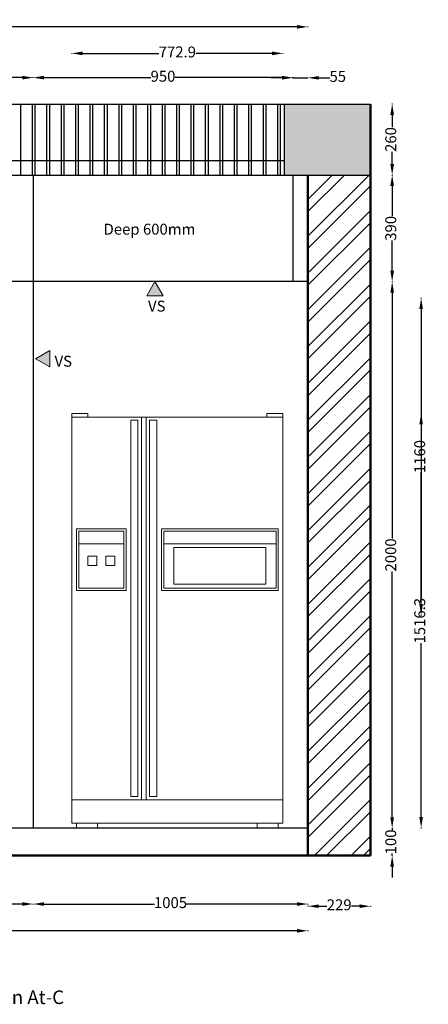
# Model space of a CAD drawing. Units: millimetres. Extents: x 2054 to 5837, y -782 to 2821.
# Tile 2 of 2: x 4342 to 5837, y -782 to 2821. Entities that reach past the tile are written whole.
import ezdxf

# ---------------------------------------------------------------- set-up
doc = ezdxf.new("R2010")
doc.units = ezdxf.units.MM
for name, color, linetype, lineweight in [('A-ANNO-DIMS', 2, 'Continuous', 18), ('A-ANNO-SYMB', 1, 'Continuous', 18), ('A-ANNO-TEXT', 7, 'Continuous', 18), ('A-EQPM', 8, 'Continuous', 18), ('A-FURN', 42, 'Continuous', 25), ('A-FURN-PATT', 8, 'Continuous', 13), ('A-WALL', 7, 'Continuous', 50), ('A-WALL-PATT', 8, 'Continuous', 13)]:
    doc.layers.add(name, color=color, linetype=linetype, lineweight=lineweight)
doc.styles.get("Standard").update_dxf_attribs({"font": 'arial.ttf'})
doc.dimstyles.new('ISO-25', dxfattribs={"dimtxt": 40, "dimasz": 40, "dimexe": 1.25, "dimexo": 0.625, "dimtad": 0, "dimtxsty": 'Standard', "dimcen": 2.5, "dimclrt": 1, "dimadec": 0, "dimazin": 0, "dimtfac": 1, "dimtmove": 0, "dimatfit": 3, "dimfxl": 1, "dimfxlon": 1, "dimarcsym": 0})

# ---------------------------------------------------------------- blocks, each defined once
blk = doc.blocks.new('*D1')
at = {"layer": 'A-ANNO-DIMS', "color": 0, "lineweight": -2, "transparency": 16777216}
for p, q in [((4391.1, -414.1), (4391.1, -416.4)), ((4431.1, -415.1), (4835, -415.1)), ((5356.1, -415.1), (4952.2, -415.1)), ((5396.1, -414.1), (5396.1, -416.4))]:
    blk.add_line(p, q, dxfattribs=at)
at = {"layer": 'A-ANNO-DIMS', "color": 0, "transparency": 16777216}
for points in [[(4431.1, -408.4), (4431.1, -421.8), (4391.1, -415.1)], [(5356.1, -408.4), (5356.1, -421.8), (5396.1, -415.1)]]:
    blk.add_solid(points, dxfattribs=at)
at = {"layer": 'Defpoints', "color": 0, "transparency": 16777216}
for p in [(4391.1, -137.8), (5396.1, -137.8), (4391.1, -415.1)]:
    blk.add_point(p, dxfattribs=at)
at = {"layer": 'A-ANNO-DIMS', "color": 0, "transparency": 16777216, "insert": (4893.6, -415.1), "char_height": 40, "attachment_point": 5}
blk.add_mtext('1005', dxfattribs=at)
blk = doc.blocks.new('*D2')
at = {"layer": 'A-ANNO-DIMS', "color": 0, "lineweight": -2, "transparency": 16777216}
for p, q in [((3941.1, -414.1), (3941.1, -416.4)), ((3981.1, -415.1), (4120.6, -415.1)), ((4351.1, -415.1), (4211.7, -415.1)), ((4391.1, -414.1), (4391.1, -416.4))]:
    blk.add_line(p, q, dxfattribs=at)
at = {"layer": 'A-ANNO-DIMS', "color": 0, "transparency": 16777216}
for points in [[(3981.1, -408.4), (3981.1, -421.8), (3941.1, -415.1)], [(4351.1, -408.4), (4351.1, -421.8), (4391.1, -415.1)]]:
    blk.add_solid(points, dxfattribs=at)
at = {"layer": 'Defpoints', "color": 0, "transparency": 16777216}
for p in [(3941.1, -137.8), (4391.1, -137.8), (3941.1, -415.1)]:
    blk.add_point(p, dxfattribs=at)
at = {"layer": 'A-ANNO-DIMS', "color": 0, "transparency": 16777216, "insert": (4166.1, -415.1), "char_height": 40, "attachment_point": 5}
blk.add_mtext('450', dxfattribs=at)
blk = doc.blocks.new('*D6')
at = {"layer": 'A-ANNO-DIMS', "color": 0, "lineweight": -2, "transparency": 16777216}
for p, q in [((2549.1, -512.1), (2549.1, -514.3)), ((2589.1, -513.1), (3911.9, -513.1)), ((5356.1, -513.1), (4033.3, -513.1)), ((5396.1, -512.1), (5396.1, -514.3))]:
    blk.add_line(p, q, dxfattribs=at)
at = {"layer": 'A-ANNO-DIMS', "color": 0, "transparency": 16777216}
for points in [[(2589.1, -506.4), (2589.1, -519.7), (2549.1, -513.1)], [(5356.1, -506.4), (5356.1, -519.7), (5396.1, -513.1)]]:
    blk.add_solid(points, dxfattribs=at)
at = {"layer": 'Defpoints', "color": 0, "transparency": 16777216}
for p in [(2549.1, -237.8), (5396.1, -237.8), (5396.1, -513.1)]:
    blk.add_point(p, dxfattribs=at)
at = {"layer": 'A-ANNO-DIMS', "color": 0, "transparency": 16777216, "insert": (3972.6, -513.1), "char_height": 40, "attachment_point": 5}
blk.add_mtext('2847', dxfattribs=at)
blk = doc.blocks.new('*D7')
at = {"layer": 'A-ANNO-DIMS', "color": 0, "lineweight": -2, "transparency": 16777216}
for p, q in [((5704.4, -97.8), (5704.4, -57.8)), ((5703.4, -137.8), (5705.6, -137.8)), ((5704.4, -137.8), (5704.4, -144.9)), ((5703.4, -237.8), (5705.6, -237.8)), ((5704.4, -237.8), (5704.4, -230.7)), ((5704.4, -277.8), (5704.4, -317.8))]:
    blk.add_line(p, q, dxfattribs=at)
at = {"layer": 'A-ANNO-DIMS', "color": 0, "transparency": 16777216}
for points in [[(5697.7, -97.8), (5711, -97.8), (5704.4, -137.8)], [(5697.7, -277.8), (5711, -277.8), (5704.4, -237.8)]]:
    blk.add_solid(points, dxfattribs=at)
at = {"layer": 'Defpoints', "color": 0, "transparency": 16777216}
for p in [(5396.1, -137.8), (5396.1, -237.8), (5704.4, -237.8)]:
    blk.add_point(p, dxfattribs=at)
at = {"layer": 'A-ANNO-DIMS', "color": 0, "transparency": 16777216, "insert": (5704.4, -187.8), "char_height": 40, "attachment_point": 5, "rotation": 90}
blk.add_mtext('100', dxfattribs=at)
blk = doc.blocks.new('*D8')
at = {"layer": 'A-ANNO-DIMS', "color": 0, "lineweight": -2, "transparency": 16777216}
for p, q in [((5703.4, 1862.2), (5705.6, 1862.2)), ((5704.4, 1822.2), (5704.4, 922.8)), ((5704.4, -97.8), (5704.4, 801.6)), ((5703.4, -137.8), (5705.6, -137.8))]:
    blk.add_line(p, q, dxfattribs=at)
at = {"layer": 'A-ANNO-DIMS', "color": 0, "transparency": 16777216}
for points in [[(5697.7, 1822.2), (5711, 1822.2), (5704.4, 1862.2)], [(5697.7, -97.8), (5711, -97.8), (5704.4, -137.8)]]:
    blk.add_solid(points, dxfattribs=at)
at = {"layer": 'Defpoints', "color": 0, "transparency": 16777216}
for p in [(5396.1, 1862.2), (5704.4, 1862.2), (5396.1, -137.8)]:
    blk.add_point(p, dxfattribs=at)
at = {"layer": 'A-ANNO-DIMS', "color": 0, "transparency": 16777216, "insert": (5704.4, 862.2), "char_height": 40, "attachment_point": 5, "rotation": 90}
blk.add_mtext('2000', dxfattribs=at)
blk = doc.blocks.new('*D9')
at = {"layer": 'A-ANNO-DIMS', "color": 0, "lineweight": -2, "transparency": 16777216}
for p, q in [((5703.4, 2252.2), (5705.6, 2252.2)), ((5704.4, 2212.2), (5704.4, 2101.9)), ((5704.4, 1902.2), (5704.4, 2012.5)), ((5703.4, 1862.2), (5705.6, 1862.2))]:
    blk.add_line(p, q, dxfattribs=at)
at = {"layer": 'A-ANNO-DIMS', "color": 0, "transparency": 16777216}
for points in [[(5697.7, 2212.2), (5711, 2212.2), (5704.4, 2252.2)], [(5697.7, 1902.2), (5711, 1902.2), (5704.4, 1862.2)]]:
    blk.add_solid(points, dxfattribs=at)
at = {"layer": 'Defpoints', "color": 0, "transparency": 16777216}
for p in [(5625.1, 2252.2), (5704.4, 2252.2), (5396.1, 1862.2)]:
    blk.add_point(p, dxfattribs=at)
at = {"layer": 'A-ANNO-DIMS', "color": 0, "transparency": 16777216, "insert": (5704.4, 2057.2), "char_height": 40, "attachment_point": 5, "rotation": 90}
blk.add_mtext('390', dxfattribs=at)
blk = doc.blocks.new('*D10')
at = {"layer": 'A-ANNO-DIMS', "color": 0, "lineweight": -2, "transparency": 16777216}
for p, q in [((5703.4, 2512.2), (5705.6, 2512.2)), ((5704.4, 2472.2), (5704.4, 2427.3)), ((5704.4, 2292.2), (5704.4, 2337.1)), ((5703.4, 2252.2), (5705.6, 2252.2))]:
    blk.add_line(p, q, dxfattribs=at)
at = {"layer": 'A-ANNO-DIMS', "color": 0, "transparency": 16777216}
for points in [[(5697.7, 2472.2), (5711, 2472.2), (5704.4, 2512.2)], [(5697.7, 2292.2), (5711, 2292.2), (5704.4, 2252.2)]]:
    blk.add_solid(points, dxfattribs=at)
at = {"layer": 'Defpoints', "color": 0, "transparency": 16777216}
for p in [(5625.1, 2512.2), (5704.4, 2512.2), (5625.1, 2252.2)]:
    blk.add_point(p, dxfattribs=at)
at = {"layer": 'A-ANNO-DIMS', "color": 0, "transparency": 16777216, "insert": (5704.4, 2382.2), "char_height": 40, "attachment_point": 5, "rotation": 90}
blk.add_mtext('260', dxfattribs=at)
blk = doc.blocks.new('*D11')
at = {"layer": 'A-ANNO-DIMS', "color": 0, "lineweight": -2, "transparency": 16777216}
for p, q in [((5301.1, 2608), (5261.1, 2608)), ((5341.1, 2607), (5341.1, 2609.2)), ((5341.1, 2608), (5396.1, 2608)), ((5396.1, 2607), (5396.1, 2609.2)), ((5436.1, 2608), (5476.1, 2608))]:
    blk.add_line(p, q, dxfattribs=at)
at = {"layer": 'A-ANNO-DIMS', "color": 0, "transparency": 16777216}
for points in [[(5301.1, 2614.6), (5301.1, 2601.3), (5341.1, 2608)], [(5436.1, 2614.6), (5436.1, 2601.3), (5396.1, 2608)]]:
    blk.add_solid(points, dxfattribs=at)
at = {"layer": 'Defpoints', "color": 0, "transparency": 16777216}
for p in [(5396.1, 2608), (5341.1, 2252.2), (5396.1, 2252.2)]:
    blk.add_point(p, dxfattribs=at)
at = {"layer": 'A-ANNO-DIMS', "color": 0, "transparency": 16777216, "insert": (5505.5, 2608), "char_height": 40, "attachment_point": 5}
blk.add_mtext('55', dxfattribs=at)
blk = doc.blocks.new('*D12')
at = {"layer": 'A-ANNO-DIMS', "color": 0, "lineweight": -2, "transparency": 16777216}
for p, q in [((4391.1, 2607.6), (4391.1, 2609.9)), ((4431.1, 2608.6), (4821.4, 2608.6)), ((5301.1, 2608.6), (4910.9, 2608.6)), ((5341.1, 2607.6), (5341.1, 2609.9))]:
    blk.add_line(p, q, dxfattribs=at)
at = {"layer": 'A-ANNO-DIMS', "color": 0, "transparency": 16777216}
for points in [[(4431.1, 2615.3), (4431.1, 2602), (4391.1, 2608.6)], [(5301.1, 2615.3), (5301.1, 2602), (5341.1, 2608.6)]]:
    blk.add_solid(points, dxfattribs=at)
at = {"layer": 'Defpoints', "color": 0, "transparency": 16777216}
for p in [(4391.1, 2608.6), (4391.1, 2252.2), (5341.1, 2252.2)]:
    blk.add_point(p, dxfattribs=at)
at = {"layer": 'A-ANNO-DIMS', "color": 0, "transparency": 16777216, "insert": (4866.1, 2608.6), "char_height": 40, "attachment_point": 5}
blk.add_mtext('950', dxfattribs=at)
blk = doc.blocks.new('*D13')
at = {"layer": 'A-ANNO-DIMS', "color": 0, "lineweight": -2, "transparency": 16777216}
for p, q in [((3941.1, 2607.6), (3941.1, 2609.9)), ((3981.1, 2608.6), (4120.6, 2608.6)), ((4351.1, 2608.6), (4211.7, 2608.6)), ((4391.1, 2607.6), (4391.1, 2609.9))]:
    blk.add_line(p, q, dxfattribs=at)
at = {"layer": 'A-ANNO-DIMS', "color": 0, "transparency": 16777216}
for points in [[(3981.1, 2615.3), (3981.1, 2602), (3941.1, 2608.6)], [(4351.1, 2615.3), (4351.1, 2602), (4391.1, 2608.6)]]:
    blk.add_solid(points, dxfattribs=at)
at = {"layer": 'Defpoints', "color": 0, "transparency": 16777216}
for p in [(3941.1, 2608.6), (3941.1, 2252.2), (4391.1, 2252.2)]:
    blk.add_point(p, dxfattribs=at)
at = {"layer": 'A-ANNO-DIMS', "color": 0, "transparency": 16777216, "insert": (4166.1, 2608.6), "char_height": 40, "attachment_point": 5}
blk.add_mtext('450', dxfattribs=at)
blk = doc.blocks.new('*D18')
at = {"layer": 'A-ANNO-DIMS', "color": 0, "lineweight": -2, "transparency": 16777216}
for p, q in [((2549.1, 2793.4), (2549.1, 2795.7)), ((2589.1, 2794.4), (3911.9, 2794.4)), ((5356.1, 2794.4), (4033.3, 2794.4)), ((5396.1, 2793.4), (5396.1, 2795.7))]:
    blk.add_line(p, q, dxfattribs=at)
at = {"layer": 'A-ANNO-DIMS', "color": 0, "transparency": 16777216}
for points in [[(2589.1, 2801.1), (2589.1, 2787.8), (2549.1, 2794.4)], [(5356.1, 2801.1), (5356.1, 2787.8), (5396.1, 2794.4)]]:
    blk.add_solid(points, dxfattribs=at)
at = {"layer": 'Defpoints', "color": 0, "transparency": 16777216}
for p in [(5396.1, 2794.4), (2549.1, 2306), (5396.1, 2252.2)]:
    blk.add_point(p, dxfattribs=at)
at = {"layer": 'A-ANNO-DIMS', "color": 0, "transparency": 16777216, "insert": (3972.6, 2794.4), "char_height": 40, "attachment_point": 5}
blk.add_mtext('2847', dxfattribs=at)
blk = doc.blocks.new('7')
at = {"color": 0}
for p, q in [((4545.85, 14047.67), (4636.65, 14047.67)), ((4545.85, 13873.04), (4545.85, 14047.67)), ((4575.8, 14047.67), (4575.8, 13883.04)), ((4577.8, 14047.67), (4577.8, 13883.04)), ((4636.65, 13873.04), (4636.65, 14047.67)), ((4548.85, 13998.66), (4568.22, 13998.66)), ((4548.85, 13974.04), (4548.85, 13998.66)), ((4568.22, 13998.66), (4568.22, 13974.04)), ((4548.85, 13993.2), (4568.22, 13993.2)), ((4585.39, 13993.2), (4633.65, 13993.2)), ((4568.22, 13974.04), (4548.85, 13974.04)), ((4545.85, 13883.04), (4636.65, 13883.04)), ((4529.28, 13871.04), (4646.15, 13871.04)), ((4545.85, 13873.04), (4636.65, 13873.04)), ((4547.85, 13871.04), (4547.85, 13873.04)), ((4547.85, 13871.04), (4556.94, 13871.04)), ((4556.94, 13871.04), (4556.94, 13873.04)), ((4625.56, 13871.04), (4625.56, 13873.04)), ((4625.56, 13871.04), (4634.65, 13871.04)), ((4634.65, 13871.04), (4634.65, 13873.04))]:
    blk.add_line(p, q, dxfattribs=at)
for points in [[(4545.85, 14047.67), (4552.73, 14047.67), (4552.73, 14049.18), (4545.85, 14049.18)], [(4636.65, 14047.67), (4629.77, 14047.67), (4629.77, 14049.18), (4636.65, 14049.18)], [(4571.22, 14046.31), (4574.26, 14046.31), (4574.26, 13884.52), (4571.22, 13884.52)], [(4582.39, 14046.31), (4579.35, 14046.31), (4579.35, 13884.52), (4582.39, 13884.52)], [(4547.85, 13973.04), (4547.85, 13999.66), (4569.22, 13999.66), (4569.22, 13973.04)], [(4634.65, 13999.66), (4584.39, 13999.66), (4584.39, 13973.04), (4634.65, 13973.04)], [(4633.65, 13998.66), (4585.39, 13998.66), (4585.39, 13974.04), (4633.65, 13974.04)], [(4629.24, 13991.57), (4589.8, 13991.57), (4589.8, 13975.77), (4629.24, 13975.77)], [(4552.72, 13987.81), (4556.6, 13987.81), (4556.6, 13983.82), (4552.72, 13983.82)], [(4560.47, 13987.81), (4564.35, 13987.81), (4564.35, 13983.82), (4560.47, 13983.82)]]:
    blk.add_lwpolyline(points, close=True, dxfattribs=at)
blk = doc.blocks.new('VS-MARKER')
h = blk.add_hatch(color=256)
h.dxf.hatch_style = 1
h.paths.add_polyline_path([(0, 0), (60, 0), (30, 52)])
blk.add_lwpolyline([(0, 0), (60, 0), (30, 52), (0, 0)])
blk = doc.blocks.new('*D28')
at = {"layer": 'A-ANNO-DIMS', "color": 0, "lineweight": -2, "transparency": 16777216}
for p, q in [((4532.1, 2696.4), (4532.1, 2698.7)), ((4572.1, 2697.4), (4850.6, 2697.4)), ((5265.1, 2697.4), (4986.6, 2697.4)), ((5305.1, 2696.4), (5305.1, 2698.7))]:
    blk.add_line(p, q, dxfattribs=at)
at = {"layer": 'A-ANNO-DIMS', "color": 0, "transparency": 16777216}
for points in [[(4572.1, 2704.1), (4572.1, 2690.8), (4532.1, 2697.4)], [(5265.1, 2704.1), (5265.1, 2690.8), (5305.1, 2697.4)]]:
    blk.add_solid(points, dxfattribs=at)
at = {"layer": 'Defpoints', "color": 0, "transparency": 16777216}
for p in [(5305.1, 2697.4), (4532.1, 1379.7), (5305.1, 1379.7)]:
    blk.add_point(p, dxfattribs=at)
at = {"layer": 'A-ANNO-DIMS', "color": 1, "transparency": 16777216, "insert": (4918.6, 2697.4), "char_height": 40, "attachment_point": 5}
blk.add_mtext('772.9', dxfattribs=at)
blk = doc.blocks.new('*D29')
at = {"layer": 'A-ANNO-DIMS', "color": 0, "lineweight": -2, "transparency": 16777216}
for p, q in [((5809.4, 1379.7), (5811.6, 1379.7)), ((5810.4, 1339.7), (5810.4, 703.4)), ((5810.4, -96.5), (5810.4, 539.8)), ((5809.4, -136.5), (5811.6, -136.5))]:
    blk.add_line(p, q, dxfattribs=at)
at = {"layer": 'A-ANNO-DIMS', "color": 0, "transparency": 16777216}
for points in [[(5803.7, 1339.7), (5817, 1339.7), (5810.4, 1379.7)], [(5803.7, -96.5), (5817, -96.5), (5810.4, -136.5)]]:
    blk.add_solid(points, dxfattribs=at)
at = {"layer": 'Defpoints', "color": 0, "transparency": 16777216}
for p in [(5305.1, 1379.7), (5810.4, 1379.7), (5288, -136.5)]:
    blk.add_point(p, dxfattribs=at)
at = {"layer": 'A-ANNO-DIMS', "color": 1, "transparency": 16777216, "insert": (5810.4, 621.6), "char_height": 40, "attachment_point": 5, "rotation": 90}
blk.add_mtext('1516.3', dxfattribs=at)
blk = doc.blocks.new('*D31')
at = {"layer": 'A-ANNO-DIMS', "color": 0, "lineweight": -2, "transparency": 16777216}
for p, q in [((5396.1, -422.1), (5396.1, -424.3)), ((5436.1, -423.1), (5465.4, -423.1)), ((5585.1, -423.1), (5555.8, -423.1)), ((5625.1, -422.1), (5625.1, -424.3))]:
    blk.add_line(p, q, dxfattribs=at)
at = {"layer": 'A-ANNO-DIMS', "color": 0, "transparency": 16777216}
for points in [[(5436.1, -416.4), (5436.1, -429.7), (5396.1, -423.1)], [(5585.1, -416.4), (5585.1, -429.7), (5625.1, -423.1)]]:
    blk.add_solid(points, dxfattribs=at)
at = {"layer": 'Defpoints', "color": 0, "transparency": 16777216}
for p in [(5396.1, -237.8), (5625.1, -237.8), (5625.1, -423.1)]:
    blk.add_point(p, dxfattribs=at)
at = {"layer": 'A-ANNO-DIMS', "color": 1, "transparency": 16777216, "insert": (5510.6, -423.1), "char_height": 40, "attachment_point": 5}
blk.add_mtext('229', dxfattribs=at)
blk = doc.blocks.new('*D32')
at = {"layer": 'A-ANNO-DIMS', "color": 0, "lineweight": -2, "transparency": 16777216}
for p, q in [((5809.4, 1802.2), (5811.6, 1802.2)), ((5810.4, 1762.2), (5810.4, 1280.6)), ((5810.4, 682.2), (5810.4, 1163.8)), ((5809.4, 642.2), (5811.6, 642.2))]:
    blk.add_line(p, q, dxfattribs=at)
at = {"layer": 'A-ANNO-DIMS', "color": 0, "transparency": 16777216}
for points in [[(5803.7, 1762.2), (5817, 1762.2), (5810.4, 1802.2)], [(5803.7, 682.2), (5817, 682.2), (5810.4, 642.2)]]:
    blk.add_solid(points, dxfattribs=at)
at = {"layer": 'Defpoints', "color": 0, "transparency": 16777216}
for p in [(3921.1, 1802.2), (5810.4, 1802.2), (3921.1, 642.2)]:
    blk.add_point(p, dxfattribs=at)
at = {"layer": 'A-ANNO-DIMS', "color": 1, "transparency": 16777216, "insert": (5810.4, 1222.2), "char_height": 40, "attachment_point": 5, "rotation": 90}
blk.add_mtext('1160', dxfattribs=at)

msp = doc.modelspace()

# ---------------------------------------------------------------- hatches: boundary and pattern name
at = {"layer": 'A-FURN-PATT'}
h = msp.add_hatch(dxfattribs=at)
h.set_pattern_fill('AR-CONC', color=256, scale=0.5)
h.paths.add_polyline_path([(2699.109, 2512.19), (2320.109, 2512.19), (2320.109, 2306.028), (2699.109, 2306.028)])
h.paths.add_polyline_path([(5625.109, 2512.19), (5310.109, 2512.19), (5310.109, 2252.19), (5625.109, 2252.19)])
at = {"layer": 'A-WALL-PATT'}
h = msp.add_hatch(dxfattribs=at)
h.set_pattern_fill('ANSI32', color=256, scale=10)
h.paths.add_polyline_path([(2549.109, 2306.028), (2320.109, 2306.028), (2320.109, -237.81), (2549.109, -237.81), (2549.109, 582.19), (2549.109, 622.19), (2549.109, 1222.19)])
h.paths.add_polyline_path([(5625.109, 2252.19), (5396.109, 2252.19), (5396.109, 1862.19), (5396.109, -237.81), (5625.109, -237.81)])

# ---------------------------------------------------------------- linework, layer by layer
at = {"layer": 'A-FURN'}
for p, q in [((2699.109, 2512.19), (5310.109, 2512.19)), ((4344.882, 2512.19), (4344.882, 2252.19)), ((4387.648, 2512.19), (4387.648, 2252.19)), ((4397.648, 2512.19), (4397.648, 2252.19)), ((4440.415, 2512.19), (4440.415, 2252.19)), ((4450.415, 2512.19), (4450.415, 2252.19)), ((4493.182, 2512.19), (4493.182, 2252.19)), ((4503.182, 2512.19), (4503.182, 2252.19)), ((4545.949, 2512.19), (4545.949, 2252.19)), ((4555.949, 2512.19), (4555.949, 2252.19)), ((4598.716, 2512.19), (4598.716, 2252.19)), ((4608.716, 2512.19), (4608.716, 2252.19)), ((4651.483, 2512.19), (4651.483, 2252.19)), ((4661.483, 2512.19), (4661.483, 2252.19)), ((4704.25, 2512.19), (4704.25, 2252.19)), ((4714.25, 2512.19), (4714.25, 2252.19)), ((4757.016, 2512.19), (4757.016, 2252.19)), ((4767.016, 2512.19), (4767.016, 2252.19)), ((4809.783, 2512.19), (4809.783, 2252.19)), ((4819.783, 2512.19), (4819.783, 2252.19)), ((4862.55, 2512.19), (4862.55, 2252.19)), ((4872.55, 2512.19), (4872.55, 2252.19)), ((4915.317, 2512.19), (4915.317, 2252.19)), ((4925.317, 2512.19), (4925.317, 2252.19)), ((4968.084, 2512.19), (4968.084, 2252.19)), ((4978.084, 2512.19), (4978.084, 2252.19)), ((5020.851, 2512.19), (5020.851, 2252.19)), ((5030.851, 2512.19), (5030.851, 2252.19)), ((5073.617, 2512.19), (5073.617, 2252.19)), ((5083.617, 2512.19), (5083.617, 2252.19)), ((5126.384, 2512.19), (5126.384, 2252.19)), ((5136.384, 2512.19), (5136.384, 2252.19)), ((5179.151, 2512.19), (5179.151, 2252.19)), ((5189.151, 2512.19), (5189.151, 2252.19)), ((5231.918, 2512.19), (5231.918, 2252.19)), ((5241.918, 2512.19), (5241.918, 2252.19)), ((5284.685, 2512.19), (5284.685, 2252.19)), ((5294.685, 2512.19), (5294.685, 2252.19)), ((5310.109, 2252.19), (5310.109, 2512.19)), ((5310.109, 2512.19), (5625.109, 2512.19)), ((2699.109, 2306.028), (5310.109, 2306.028)), ((2549.109, 2252.19), (5310.109, 2252.19)), ((4391.109, 2252.19), (4391.109, 1862.19)), ((5310.109, 2252.19), (5625.109, 2252.19)), ((5341.109, 2252.19), (5341.109, 1862.19)), ((5396.109, 1862.19), (3941.109, 1862.19)), ((4391.109, 1862.19), (4391.109, -137.81)), ((5396.109, -137.81), (2549.109, -137.81))]:
    msp.add_line(p, q, dxfattribs=at)
at = {"layer": 'A-WALL'}
for p, q in [((5625.109, 2512.19), (5625.109, 2252.19)), ((5396.109, 2252.19), (5396.109, 1862.19)), ((5625.109, 2252.19), (5625.109, -237.81)), ((5396.109, 1862.19), (5396.109, -237.81)), ((5625.109, -237.81), (2320.109, -237.81))]:
    msp.add_line(p, q, dxfattribs=at)

# ---------------------------------------------------------------- block references
at = {"layer": 'A-ANNO-SYMB'}
msp.add_blockref('VS-MARKER', (4806.426, 1810.229), dxfattribs=at)
at = {"layer": 'A-ANNO-SYMB', "rotation": 90.0000000000013}
msp.add_blockref('VS-MARKER', (4451.731, 1550.184), dxfattribs=at)
at = {"layer": 'A-EQPM', "xscale": 8.511705981434162, "yscale": 8.511705981434162, "zscale": 8.511705981434162}
msp.add_blockref('7', (-34160.78, -118202.758), dxfattribs=at)

# ---------------------------------------------------------------- texts
at = {"layer": 'A-ANNO-SYMB', "attachment_point": 1}
for s, width, insert, char_height in [('VS', 129.91792, (4811.338, 1792.597), 40), ('VS', 129.91792, (4469.401, 1590.944), 40), ('{Kitchen Elevation At-C}', 1817.98967, (3796.43, -731.1), 50)]:
    msp.add_mtext_dynamic_manual_height_columns(s, width=width, gutter_width=12.5, heights=[0], dxfattribs=dict(at, insert=insert, char_height=char_height))
at = {"layer": 'A-ANNO-TEXT', "insert": (4648.688, 2074.157), "char_height": 40, "attachment_point": 1}
msp.add_mtext_dynamic_manual_height_columns('{Deep 600mm}', width=408.10443, gutter_width=12.5, heights=[0], dxfattribs=at)

# ---------------------------------------------------------------- dimensions: what is measured, and where the dimension line sits
at = {"layer": 'A-ANNO-DIMS'}
for base, p1, p2, override, picture, middle in [((5396.109, 2794.425), (2549.109, 2306.028), (5396.109, 2252.19), {"dimclrd": 0, "dimclre": 0, "dimclrt": 0}, '*D18', (3972.609, 2794.425)), ((5305.051, 2697.44), (4532.145, 1379.722), (5305.051, 1379.722), {"dimdec": 1, "dimlfac": 1, "dimrnd": 0, "dimzin": 0, "dimdsep": 46, "dimlunit": 2}, '*D28', (4918.598, 2697.44)), ((3941.109, 2608.643), (4391.109, 2252.19), (3941.109, 2252.19), {"dimclrd": 0, "dimclre": 0, "dimclrt": 0, "dimtmove": 1}, '*D13', (4166.109, 2608.643)), ((4391.109, 2608.643), (5341.109, 2252.19), (4391.109, 2252.19), {"dimclrd": 0, "dimclre": 0, "dimclrt": 0}, '*D12', (4866.109, 2608.643)), ((5396.109, 2607.974), (5341.109, 2252.19), (5396.109, 2252.19), {"dimclrd": 0, "dimclre": 0, "dimclrt": 0}, '*D11', (5505.534, 2607.974)), ((3941.109, -415.115), (4391.109, -137.81), (3941.109, -137.81), {"dimclrd": 0, "dimclre": 0, "dimclrt": 0, "dimtmove": 1}, '*D2', (4166.109, -415.115)), ((4391.109, -415.115), (5396.109, -137.81), (4391.109, -137.81), {"dimclrd": 0, "dimclre": 0, "dimclrt": 0}, '*D1', (4893.609, -415.115)), ((5396.109, -513.067), (2549.109, -237.81), (5396.109, -237.81), {"dimclrd": 0, "dimclre": 0, "dimclrt": 0}, '*D6', (3972.609, -513.067)), ((5625.109, -423.06), (5396.109, -237.81), (5625.109, -237.81), {"dimdec": 0, "dimlfac": 1, "dimrnd": 0, "dimzin": 0, "dimdsep": 46, "dimlunit": 2}, '*D31', (5510.609, -423.06))]:
    dim = msp.add_linear_dim(base=base, p1=p1, p2=p2, dimstyle='ISO-25', override=override, dxfattribs=at)
    dim.commit()
    dim.dimension.update_dxf_attribs({"geometry": picture, "text_midpoint": middle})
for base, p1, p2, override, picture, middle in [((5704.353, 2512.19), (5625.109, 2252.19), (5625.109, 2512.19), {"dimclrd": 0, "dimclre": 0, "dimclrt": 0, "dimtmove": 1}, '*D10', (5704.353, 2382.19)), ((5704.353, 2252.19), (5396.109, 1862.19), (5625.109, 2252.19), {"dimclrd": 0, "dimclre": 0, "dimclrt": 0, "dimtmove": 1}, '*D9', (5704.353, 2057.19)), ((5704.353, 1862.19), (5396.109, -137.81), (5396.109, 1862.19), {"dimclrd": 0, "dimclre": 0, "dimclrt": 0}, '*D8', (5704.353, 862.19)), ((5810.359, 1802.19), (3921.109, 642.19), (3921.109, 1802.19), {"dimdec": 0, "dimlfac": 1, "dimrnd": 0, "dimzin": 0, "dimdsep": 46, "dimlunit": 2}, '*D32', (5810.359, 1222.19)), ((5810.359, 1379.722), (5288.027, -136.538), (5305.051, 1379.722), {"dimdec": 1, "dimlfac": 1, "dimrnd": 0, "dimzin": 0, "dimdsep": 46, "dimlunit": 2}, '*D29', (5810.359, 621.592)), ((5704.353, -237.81), (5396.109, -137.81), (5396.109, -237.81), {"dimclrd": 0, "dimclre": 0, "dimclrt": 0}, '*D7', (5704.353, -187.81))]:
    dim = msp.add_linear_dim(base=base, p1=p1, p2=p2, angle=90, dimstyle='ISO-25', override=override, dxfattribs=at)
    dim.commit()
    dim.dimension.update_dxf_attribs({"geometry": picture, "text_midpoint": middle})

doc.saveas('drawing.dxf')
